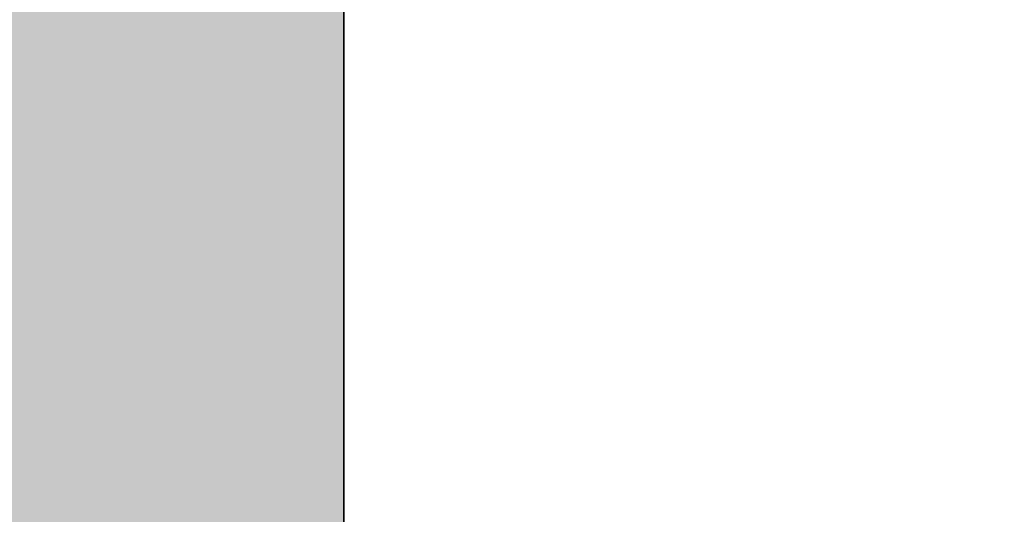
# Model space of a CAD drawing. Units: inches. Extents: x 2696 to 3240, y 1564 to 2310.
# Tile 5 of 76: x 2893.424 to 2903.397, y 1633.529 to 1638.544. Entities that reach past the tile are written whole.
import ezdxf

# ---------------------------------------------------------------- set-up
doc = ezdxf.new("R2010")
doc.units = ezdxf.units.IN
for name, color, linetype, lineweight in [('A-ANNO-DIMS', 3, 'Continuous', 18), ('A-WALL', 7, 'Continuous', 35), ('A-WALL-PATT', 9, 'Continuous', 13)]:
    doc.layers.add(name, color=color, linetype=linetype, lineweight=lineweight)
doc.styles.add('TIMES NEW', font='times.ttf')
doc.dimstyles.new('Siddhuu', dxfattribs={"dimtxt": 6, "dimasz": 2.5, "dimexe": 1.25, "dimexo": 0.625, "dimtad": 1, "dimdec": 1, "dimlunit": 4, "dimtxsty": 'TIMES NEW', "dimcen": 2.5, "dimclrd": 256, "dimclre": 1, "dimclrt": 7, "dimadec": 0, "dimazin": 0, "dimtfac": 1, "dimtdec": 1, "dimtmove": 0, "dimatfit": 3, "dimfxl": 1, "dimtolj": 1, "dimlwd": -1, "dimarcsym": 0})

# ---------------------------------------------------------------- blocks, each defined once
blk = doc.blocks.new('*D36')
at = {"layer": 'A-ANNO-DIMS', "color": 1, "lineweight": -2, "transparency": 16777216}
for p, q in [((3008.2374, 1629.3861), (3008.2374, 1619.4611)), ((3070.2374, 1629.3861), (3070.2374, 1619.4611))]:
    blk.add_line(p, q, dxfattribs=at)
at = {"layer": 'A-ANNO-DIMS', "transparency": 16777216}
for p, q in [((3008.2374, 1620.7111), (2894.7181, 1620.7111)), ((3067.7374, 1620.7111), (3010.7374, 1620.7111))]:
    blk.add_line(p, q, dxfattribs=at)
for points in [[(3010.7374, 1621.1278), (3010.7374, 1620.2944), (3008.2374, 1620.7111)], [(3067.7374, 1621.1278), (3067.7374, 1620.2944), (3070.2374, 1620.7111)]]:
    blk.add_solid(points, dxfattribs=at)
at = {"layer": 'Defpoints', "color": 0, "transparency": 16777216}
for p in [(3008.2374, 1630.0111), (3070.2374, 1630.0111), (3008.2374, 1620.7111)]:
    blk.add_point(p, dxfattribs=at)
at = {"layer": 'A-ANNO-DIMS', "color": 7, "transparency": 16777216, "insert": (2950.2277, 1624.4031), "char_height": 6, "attachment_point": 5, "style": 'TIMES NEW'}
blk.add_mtext('\\A1;BALCONY DOOR 5\'-2" TYP.', dxfattribs=at)
blk = doc.blocks.new('*D57')
at = {"layer": 'A-ANNO-DIMS', "color": 1, "lineweight": -2, "transparency": 16777216}
for p, q in [((2754.6114, 2018.5761), (2754.6114, 1568.9511)), ((2956.7088, 2018.5761), (2956.7088, 1568.9511))]:
    blk.add_line(p, q, dxfattribs=at)
at = {"layer": 'A-ANNO-DIMS', "transparency": 16777216}
blk.add_line((2757.1114, 1570.2011), (2954.2088, 1570.2011), dxfattribs=at)
for points in [[(2757.1114, 1570.6178), (2757.1114, 1569.7844), (2754.6114, 1570.2011)], [(2954.2088, 1570.6178), (2954.2088, 1569.7844), (2956.7088, 1570.2011)]]:
    blk.add_solid(points, dxfattribs=at)
at = {"layer": 'Defpoints', "color": 0, "transparency": 16777216}
for p in [(2754.6114, 2019.2011), (2956.7088, 2019.2011), (2956.7088, 1570.2011)]:
    blk.add_point(p, dxfattribs=at)
at = {"layer": 'A-ANNO-DIMS', "color": 7, "transparency": 16777216, "insert": (2855.6601, 1573.878), "char_height": 6, "attachment_point": 5, "style": 'TIMES NEW'}
blk.add_mtext('\\A1;16\'-10"', dxfattribs=at)
blk = doc.blocks.new('*D69')
at = {"layer": 'A-ANNO-DIMS', "color": 1, "lineweight": -2, "transparency": 16777216}
for p, q in [((2841.889, 2261.5761), (2841.889, 1568.9511)), ((2905.9101, 2261.5761), (2905.9101, 1568.9511))]:
    blk.add_line(p, q, dxfattribs=at)
at = {"layer": 'A-ANNO-DIMS', "transparency": 16777216}
blk.add_line((2844.389, 1570.2011), (2903.4101, 1570.2011), dxfattribs=at)
for points in [[(2844.389, 1570.6178), (2844.389, 1569.7844), (2841.889, 1570.2011)], [(2903.4101, 1570.6178), (2903.4101, 1569.7844), (2905.9101, 1570.2011)]]:
    blk.add_solid(points, dxfattribs=at)
at = {"layer": 'Defpoints', "color": 0, "transparency": 16777216}
for p in [(2841.889, 2262.2011), (2905.9101, 2262.2011), (2905.9101, 1570.2011)]:
    blk.add_point(p, dxfattribs=at)
at = {"layer": 'A-ANNO-DIMS', "color": 7, "transparency": 16777216, "insert": (2873.8995, 1573.878), "char_height": 6, "attachment_point": 5, "style": 'TIMES NEW'}
blk.add_mtext('\\A1;5\'-4"', dxfattribs=at)

msp = doc.modelspace()

# ---------------------------------------------------------------- hatches: boundary and pattern name
at = {"layer": 'A-WALL-PATT', "transparency": 33554556}
h = msp.add_hatch(color=256, dxfattribs=at)
h.dxf.hatch_style = 1
h.paths.add_polyline_path([(2879.1114, 2253.2011), (2905.9101, 2253.2011), (2905.9101, 2262.2011), (2841.889, 2262.2011), (2841.889, 2253.2011), (2870.1114, 2253.2011), (2870.1114, 2176.6011), (2965.7088, 2176.6011), (2965.7088, 2206.7011), (2973.5828, 2206.7011), (2973.5828, 2215.7011), (2965.7088, 2215.7011), (2965.7088, 2262.2011), (2929.9101, 2262.2011), (2929.9101, 2253.2011), (2956.7088, 2253.2011), (2956.7088, 2185.6011), (2879.1114, 2185.6011)])
h.paths.add_polyline_path([(2782.8338, 2262.2011), (2745.6114, 2262.2011), (2745.6114, 2228.7287), (2754.6114, 2228.7287), (2754.6114, 2253.2011), (2782.8338, 2253.2011)])
h.paths.add_polyline_path([(2754.6114, 2136.2011), (2965.7088, 2136.2011), (2965.7088, 2145.2011), (2879.1114, 2145.2011), (2879.1114, 2147.0735), (2877.3397, 2147.0735), (2870.1114, 2147.0735), (2870.1114, 2145.2011), (2754.6114, 2145.2011), (2754.6114, 2169.6735), (2745.6114, 2169.6735), (2745.6114, 2000.2011), (2754.6114, 2000.2011), (2754.6114, 2019.2011), (2849.0828, 2019.2011), (2849.0828, 2023.7011), (2841.2088, 2023.7011), (2841.2088, 2051.8271), (2836.7088, 2051.8271), (2836.7088, 2023.7011), (2754.6114, 2023.7011), (2754.6114, 2091.2011), (2836.7088, 2091.2011), (2836.7088, 2087.8271), (2841.2088, 2087.8271), (2841.2088, 2095.7011), (2754.6114, 2095.7011)])
h.paths.add_polyline_path([(2965.7088, 2136.2011), (2956.7088, 2136.2011), (2956.7088, 2023.7011), (2885.0828, 2023.7011), (2885.0828, 2019.2011), (2956.7088, 2019.2011), (2956.7088, 1950.5751), (2965.7088, 1950.5751), (2965.7088, 1980.2011), (2973.5828, 1980.2011), (2973.5828, 1989.2011), (2965.7088, 1989.2011)])
h.paths.add_polyline_path([(2754.6114, 1906.7011), (2880.2088, 1906.7011), (2884.7088, 1906.7011), (2956.7088, 1906.7011), (2956.7088, 1792.7011), (2944.7088, 1792.7011), (2944.7088, 1783.7011), (2956.7088, 1783.7011), (2956.7088, 1740.2011), (2884.7088, 1740.2011), (2884.7088, 1783.7011), (2896.7088, 1783.7011), (2896.7088, 1792.7011), (2884.7088, 1792.7011), (2884.7088, 1846.7011), (2880.2088, 1846.7011), (2880.2088, 1740.2011), (2754.6114, 1740.2011), (2754.6114, 1777.2011), (2745.6114, 1777.2011), (2745.6114, 1692.7011), (2754.6114, 1692.7011), (2754.6114, 1731.2011), (2956.7088, 1731.2011), (2956.7088, 1723.3271), (2965.7088, 1723.3271), (2965.7088, 1884.2011), (2973.5828, 1884.2011), (2973.5828, 1893.2011), (2965.7088, 1893.2011), (2965.7088, 1914.5751), (2956.7088, 1914.5751), (2956.7088, 1911.2011), (2754.6114, 1911.2011), (2754.6114, 1930.2011), (2745.6114, 1930.2011), (2745.6114, 1817.2011), (2754.6114, 1817.2011), (2754.6114, 1854.2011), (2826.6114, 1854.2011), (2826.6114, 1868.8271), (2822.1114, 1868.8271), (2822.1114, 1858.7011), (2754.6114, 1858.7011)])
h.paths.add_polyline_path([(2965.7088, 1656.2011), (3008.2374, 1656.2011), (3008.2374, 1665.2011), (2965.7088, 1665.2011), (2965.7088, 1693.3271), (2956.7088, 1693.3271), (2956.7088, 1686.2011), (2934.5828, 1686.2011), (2934.5828, 1681.7011), (2956.7088, 1681.7011), (2956.7088, 1614.2011), (2896.7088, 1614.2011), (2896.7088, 1681.7011), (2904.5828, 1681.7011), (2904.5828, 1686.2011), (2892.2088, 1686.2011), (2892.2088, 1614.2011), (2858.4101, 1614.2011), (2858.4101, 1605.2011), (2965.7088, 1605.2011)])
h.paths.add_polyline_path([(2788.4101, 1614.2011), (2754.6114, 1614.2011), (2754.6114, 1652.7011), (2745.6114, 1652.7011), (2745.6114, 1605.2011), (2788.4101, 1605.2011)])
h.paths.add_polyline_path([(3199.6114, 1633.0476), (3190.6114, 1633.0476), (3190.6114, 1614.2011), (3082.6114, 1614.2011), (3082.6114, 1665.2011), (3070.2374, 1665.2011), (3070.2374, 1656.2011), (3078.1114, 1656.2011), (3078.1114, 1605.2011), (3199.6114, 1605.2011)])
h.paths.add_polyline_path([(3199.6114, 1702.0476), (3190.6114, 1702.0476), (3190.6114, 1699.7011), (3106.6114, 1699.7011), (3106.6114, 1747.7011), (3190.6114, 1747.7011), (3190.6114, 1752.2011), (3082.6114, 1752.2011), (3082.6114, 1760.0751), (3078.1114, 1760.0751), (3078.1114, 1747.7011), (3102.1114, 1747.7011), (3102.1114, 1699.7011), (3078.1114, 1699.7011), (3078.1114, 1695.2011), (3190.6114, 1695.2011), (3190.6114, 1676.3546), (3199.6114, 1676.3546)])
h.paths.add_polyline_path([(3199.6114, 1783.2011), (3190.6114, 1783.2011), (3190.6114, 1745.3546), (3199.6114, 1745.3546)])
h.paths.add_polyline_path([(3082.6114, 1884.2011), (3190.6114, 1884.2011), (3190.6114, 1853.2011), (3199.6114, 1853.2011), (3199.6114, 1901.7011), (3190.6114, 1901.7011), (3190.6114, 1893.2011), (3005.5828, 1893.2011), (3005.5828, 1891.2811), (3005.5828, 1884.2011), (3078.1114, 1884.2011), (3078.1114, 1792.0751), (3082.6114, 1792.0751)])
h.paths.add_polyline_path([(3199.6114, 1994.7011), (3190.6114, 1994.7011), (3190.6114, 1989.2011), (3073.7088, 1989.2011), (3073.7088, 2034.2011), (3069.2088, 2034.2011), (3069.2088, 1989.2011), (3005.5828, 1989.2011), (3005.5828, 1980.2011), (3190.6114, 1980.2011), (3190.6114, 1971.7011), (3199.6114, 1971.7011)])
h.paths.add_polyline_path([(3199.6114, 2155.2011), (3190.6114, 2155.2011), (3190.6114, 2064.7011), (3199.6114, 2064.7011)])
h.paths.add_polyline_path([(3190.6114, 2074.7011), (3106.6114, 2074.7011), (3106.6114, 2122.7011), (3190.6114, 2122.7011), (3190.6114, 2127.2011), (3082.7088, 2127.2011), (3082.7088, 2135.0751), (3073.7088, 2135.0751), (3073.7088, 2122.7011), (3102.1114, 2122.7011), (3102.1114, 2074.7011), (3069.2088, 2074.7011), (3069.2088, 2070.2011), (3190.6114, 2070.2011)])
h.paths.add_polyline_path([(3082.7088, 2253.2011), (3190.6114, 2253.2011), (3190.6114, 2225.2011), (3199.6114, 2225.2011), (3199.6114, 2262.2011), (3073.7088, 2262.2011), (3073.7088, 2215.7011), (3035.5828, 2215.7011), (3035.5828, 2206.7011), (3073.7088, 2206.7011), (3073.7088, 2171.0751), (3082.7088, 2171.0751)])

# ---------------------------------------------------------------- linework, layer by layer
at = {"layer": 'A-WALL'}
msp.add_line((2896.7088, 1681.7011), (2896.7088, 1614.2011), dxfattribs=at)

# ---------------------------------------------------------------- dimensions: what is measured, and where the dimension line sits
at = {"layer": 'A-ANNO-DIMS'}
for base, p1, p2, picture, middle in [((2905.9101, 1570.2011), (2841.889, 2262.2011), (2905.9101, 2262.2011), '*D69', (2873.8995, 1573.878)), ((2956.7088, 1570.2011), (2754.6114, 2019.2011), (2956.7088, 2019.2011), '*D57', (2855.6601, 1573.878))]:
    dim = msp.add_linear_dim(base=base, p1=p1, p2=p2, dimstyle='Siddhuu', override={"dimdec": 1, "dimlfac": 1, "dimrnd": 0, "dimzin": 1, "dimdsep": 46, "dimlunit": 4, "dimfrac": 2}, dxfattribs=at)
    dim.commit()
    dim.dimension.update_dxf_attribs({"geometry": picture, "text_midpoint": middle})
dim = msp.add_linear_dim(base=(3008.2374, 1620.7111), p1=(3070.2374, 1630.0111), p2=(3008.2374, 1630.0111), angle=180, text='BALCONY DOOR <> TYP.', dimstyle='Siddhuu', override={"dimdec": 1, "dimlfac": 1, "dimrnd": 0, "dimzin": 1, "dimdsep": 46, "dimlunit": 4, "dimfrac": 2}, dxfattribs=at)
dim.commit()
dim.dimension.update_dxf_attribs({"geometry": '*D36', "text_midpoint": (2950.2277, 1624.4031)})

doc.saveas('drawing.dxf')
